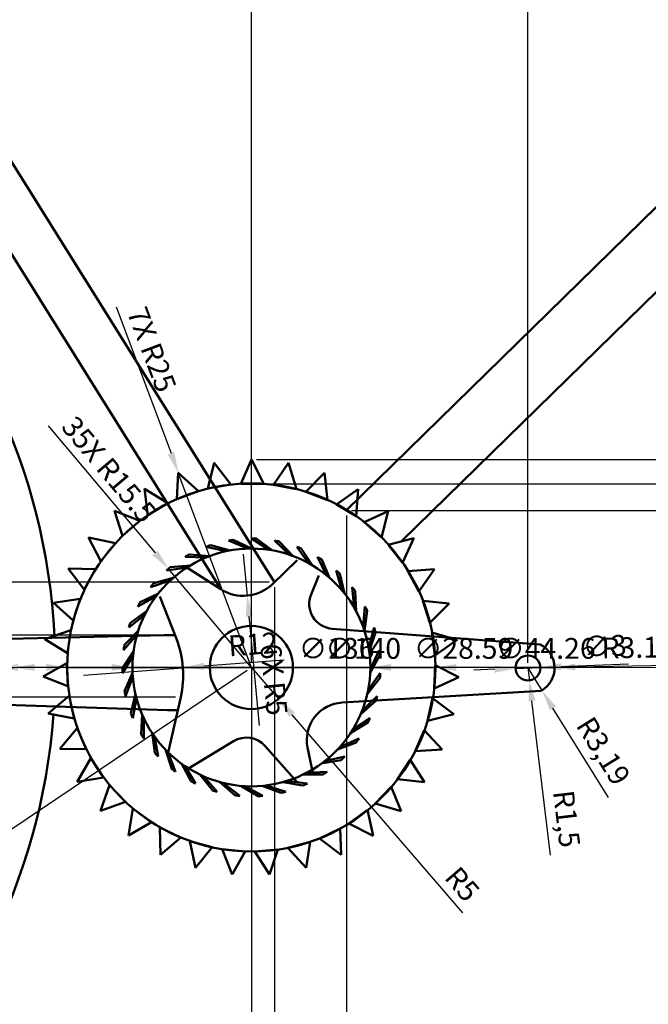
# Model space of a CAD drawing. Units: millimetres. Extents: x 1068 to 1546, y 1743 to 2032.
# Tile 4 of 9: x 1243 to 1318, y 1809 to 1928. Entities that reach past the tile are written whole.
import ezdxf

# ---------------------------------------------------------------- set-up
doc = ezdxf.new("R2010")
doc.units = ezdxf.units.MM
for name, color, linetype, lineweight in [('M-CONS', 8, 'Continuous', 18), ('M-DIMS', 2, 'Continuous', 25), ('M-OUTL', 7, 'Continuous', 50)]:
    doc.layers.add(name, color=color, linetype=linetype, lineweight=lineweight)
doc.styles.get("Standard").update_dxf_attribs({"font": 'arial.ttf'})
doc.dimstyles.new('ISO-25', dxfattribs={"dimtxt": 2.5, "dimasz": 2.5, "dimexe": 1.25, "dimexo": 0.625, "dimtad": 1, "dimtxsty": 'Standard', "dimcen": 2.5, "dimadec": 0, "dimazin": 0, "dimtfac": 1, "dimtmove": 0, "dimatfit": 3, "dimfxl": 1, "dimarcsym": 0})

# ---------------------------------------------------------------- blocks, each defined once
blk = doc.blocks.new('*U1')
for p, q in [((-1.39, -1.45), (-0.1, 1.46)), ((-0.1, 1.46), (1.39, -1.46)), ((1.39, -1.46), (-1.39, -1.45))]:
    blk.add_line(p, q)
blk = doc.blocks.new('*U2')
at = {"layer": 'M-OUTL', "color": 0, "linetype": 'ByBlock', "lineweight": -2, "transparency": 16777216}
for p, rotation in [((1266.68, 1872.95), 10.28571428571424), ((1275.09, 1872.9), 349.7142857142858), ((1262.61, 1871.85), 20.57142857142856), ((1279.15, 1871.75), 339.4285714285715), ((1258.79, 1870.04), 30.85714285714287), ((1282.94, 1869.9), 329.1428571428572), ((1255.37, 1867.58), 41.14285714285714), ((1286.34, 1867.4), 318.8571428571429), ((1252.43, 1864.54), 51.42857142857144), ((1289.24, 1864.33), 308.5714285714286), ((1250.09, 1861.04), 61.71428571428574), ((1291.54, 1860.8), 298.2857142857143), ((1248.41, 1857.16), 72.00000000000001), ((1293.18, 1856.91), 288), ((1247.44, 1853.06), 82.2857142857143), ((1294.1, 1852.79), 277.7142857142857), ((1247.23, 1848.84), 92.57142857142858), ((1294.26, 1848.57), 267.4285714285714), ((1247.77, 1844.66), 102.8571428571429), ((1293.67, 1844.39), 257.1428571428572), ((1249.05, 1840.63), 113.1428571428571), ((1292.34, 1840.39), 246.8571428571429), ((1251.03, 1836.91), 123.4285714285714), ((1290.32, 1836.68), 236.5714285714286), ((1253.64, 1833.59), 133.7142857142857), ((1287.67, 1833.4), 226.2857142857143), ((1256.81, 1830.8), 144), ((1284.48, 1830.64), 216), ((1260.42, 1828.61), 154.2857142857143), ((1280.84, 1828.5), 205.7142857142857), ((1264.36, 1827.11), 164.5714285714286), ((1268.51, 1826.33), 174.8571428571429), ((1276.88, 1827.04), 195.4285714285714), ((1272.73, 1826.31), 185.1428571428572)]:
    blk.add_blockref('*U1', p, dxfattribs=dict(at, rotation=rotation))
blk.add_blockref('*U1', (1270.89, 1873.3), dxfattribs=at)
blk = doc.blocks.new('*U3')
for p, q in [((0.05, -0.53), (-2.13, 0.52)), ((0.05, 0.68), (2.13, -0.68))]:
    blk.add_line(p, q)
blk = doc.blocks.new('*U4')
at = {"layer": 'M-OUTL', "color": 0, "linetype": 'ByBlock', "lineweight": -2, "transparency": 16777216}
for p, rotation in [((1265.53, 1863.62), 20.57142857142856), ((1268.09, 1864.34), 10.28571428571424), ((1273.38, 1864.36), 349.7142857142858), ((1275.95, 1863.66), 339.4285714285715), ((1263.14, 1862.46), 30.85714285714285), ((1278.34, 1862.51), 329.1428571428572), ((1261, 1860.89), 41.14285714285714), ((1280.5, 1860.96), 318.8571428571429), ((1259.17, 1858.96), 51.42857142857142), ((1282.34, 1859.04), 308.5714285714286), ((1257.71, 1856.74), 61.71428571428571), ((1283.81, 1856.83), 298.2857142857143), ((1256.67, 1854.29), 72), ((1284.87, 1854.39), 288), ((1285.47, 1851.8), 277.7142857142858), ((1256.09, 1851.7), 82.28571428571429), ((1255.98, 1849.05), 92.57142857142856), ((1285.6, 1849.15), 267.4285714285714), ((1256.35, 1846.41), 102.8571428571428), ((1285.25, 1846.51), 257.1428571428571), ((1257.18, 1843.89), 113.1428571428571), ((1284.44, 1843.98), 246.8571428571429), ((1258.45, 1841.55), 123.4285714285714), ((1283.19, 1841.64), 236.5714285714286), ((1260.11, 1839.48), 133.7142857142857), ((1281.54, 1839.56), 226.2857142857143), ((1262.12, 1837.74), 144), ((1279.54, 1837.8), 216), ((1264.4, 1836.39), 154.2857142857143), ((1277.26, 1836.43), 205.7142857142857), ((1266.89, 1835.46), 164.5714285714286), ((1274.78, 1835.49), 195.4285714285714), ((1269.51, 1835), 174.8571428571429), ((1272.17, 1835.01), 185.1428571428571)]:
    blk.add_blockref('*U3', p, dxfattribs=dict(at, rotation=rotation))
blk.add_blockref('*U3', (1270.74, 1864.58), dxfattribs=at)
blk = doc.blocks.new('*D5')
at = {"layer": 'Defpoints', "color": 0, "transparency": 16777216}
for p in [(1177.23, 1849.76), (1402.23, 1849.76), (1402.23, 1747.98)]:
    blk.add_point(p, dxfattribs=at)
at = {"layer": 'M-DIMS', "color": 0, "lineweight": -2, "transparency": 16777216}
for p, q in [((1177.23, 1849.14), (1177.23, 1746.73)), ((1402.23, 1849.14), (1402.23, 1746.73)), ((1179.73, 1747.98), (1399.73, 1747.98))]:
    blk.add_line(p, q, dxfattribs=at)
at = {"layer": 'M-DIMS', "color": 0, "transparency": 16777216}
for points in [[(1179.73, 1748.39), (1179.73, 1747.56), (1177.23, 1747.98)], [(1399.73, 1748.39), (1399.73, 1747.56), (1402.23, 1747.98)]]:
    blk.add_solid(points, dxfattribs=at)
at = {"layer": 'M-DIMS', "color": 0, "transparency": 16777216, "insert": (1289.73, 1749.88), "char_height": 2.5, "attachment_point": 5}
blk.add_mtext('225', dxfattribs=at)
blk = doc.blocks.new('*D6')
at = {"layer": 'Defpoints', "color": 0, "transparency": 16777216}
for p in [(1172.23, 1849.76), (1270.79, 1849.76), (1270.79, 1762.16)]:
    blk.add_point(p, dxfattribs=at)
at = {"layer": 'M-DIMS', "color": 0, "lineweight": -2, "transparency": 16777216}
for p, q in [((1172.23, 1849.14), (1172.23, 1760.91)), ((1270.79, 1849.14), (1270.79, 1760.91)), ((1174.73, 1762.16), (1268.29, 1762.16))]:
    blk.add_line(p, q, dxfattribs=at)
at = {"layer": 'M-DIMS', "color": 0, "transparency": 16777216}
for points in [[(1174.73, 1762.57), (1174.73, 1761.74), (1172.23, 1762.16)], [(1268.29, 1762.57), (1268.29, 1761.74), (1270.79, 1762.16)]]:
    blk.add_solid(points, dxfattribs=at)
at = {"layer": 'M-DIMS', "color": 0, "transparency": 16777216, "insert": (1221.51, 1764.28), "char_height": 2.5, "attachment_point": 5}
blk.add_mtext('98,56', dxfattribs=at)
blk = doc.blocks.new('*D18')
at = {"layer": 'Defpoints', "color": 0, "transparency": 16777216}
for p in [(1270.79, 1849.76), (1274.05, 1845.97)]:
    blk.add_point(p, dxfattribs=at)
at = {"layer": 'M-DIMS', "color": 0, "lineweight": -2, "transparency": 16777216}
for p, q in [((1270.79, 1849.76), (1274.05, 1845.97)), ((1296.19, 1820.25), (1275.68, 1844.08))]:
    blk.add_line(p, q, dxfattribs=at)
at = {"layer": 'M-DIMS', "color": 0, "transparency": 16777216}
blk.add_solid([(1276, 1844.35), (1275.36, 1843.81), (1274.05, 1845.97)], dxfattribs=at)
at = {"layer": 'M-DIMS', "color": 0, "transparency": 16777216, "insert": (1295.89, 1823.5), "char_height": 2.5, "attachment_point": 5, "rotation": 310.7194}
blk.add_mtext('R5', dxfattribs=at)
blk = doc.blocks.new('*D19')
at = {"layer": 'Defpoints', "color": 0, "transparency": 16777216}
for p in [(1304.02, 1849.7), (1304.2, 1848.21)]:
    blk.add_point(p, dxfattribs=at)
at = {"layer": 'M-DIMS', "color": 0, "lineweight": -2, "transparency": 16777216}
for p, q in [((1304.02, 1849.7), (1304.2, 1848.21)), ((1306.74, 1827.19), (1304.5, 1845.73))]:
    blk.add_line(p, q, dxfattribs=at)
at = {"layer": 'M-DIMS', "color": 0, "transparency": 16777216}
blk.add_solid([(1304.92, 1845.78), (1304.09, 1845.68), (1304.2, 1848.21)], dxfattribs=at)
at = {"layer": 'M-DIMS', "color": 0, "transparency": 16777216, "insert": (1308.36, 1831.52), "char_height": 2.5, "attachment_point": 5, "rotation": 276.8719}
blk.add_mtext('R1,5', dxfattribs=at)
blk = doc.blocks.new('*D20')
at = {"layer": 'Defpoints', "color": 0, "transparency": 16777216}
for p in [(1304.02, 1849.7), (1305.71, 1846.99)]:
    blk.add_point(p, dxfattribs=at)
at = {"layer": 'M-DIMS', "color": 0, "lineweight": -2, "transparency": 16777216}
for p, q in [((1304.02, 1849.7), (1305.71, 1846.99)), ((1313.69, 1834.12), (1307.02, 1844.86))]:
    blk.add_line(p, q, dxfattribs=at)
at = {"layer": 'M-DIMS', "color": 0, "transparency": 16777216}
blk.add_solid([(1307.38, 1845.08), (1306.67, 1844.64), (1305.71, 1846.99)], dxfattribs=at)
at = {"layer": 'M-DIMS', "color": 0, "transparency": 16777216, "insert": (1312.82, 1839.55), "char_height": 2.5, "attachment_point": 5, "rotation": 301.802}
blk.add_mtext('R3,19', dxfattribs=at)
blk = doc.blocks.new('*D23')
at = {"layer": 'Defpoints', "color": 0, "transparency": 16777216}
for p in [(1170.51, 1998.5), (1125.92, 1968.44), (1270.79, 1849.76)]:
    blk.add_point(p, dxfattribs=at)
at = {"layer": 'M-DIMS', "color": 0, "lineweight": -2, "transparency": 16777216}
for p, q in [((1169.99, 1998.15), (1124.89, 1967.74)), ((1224.8, 1821.77), (1127.32, 1966.36)), ((1270.27, 1849.41), (1225.16, 1819))]:
    blk.add_line(p, q, dxfattribs=at)
at = {"layer": 'M-DIMS', "color": 0, "transparency": 16777216}
for points in [[(1127.67, 1966.6), (1126.98, 1966.13), (1125.92, 1968.44)], [(1225.15, 1822.01), (1224.45, 1821.54), (1226.2, 1819.7)]]:
    blk.add_solid(points, dxfattribs=at)
at = {"layer": 'M-DIMS', "color": 0, "transparency": 16777216, "insert": (1177.82, 1895.26), "char_height": 2.5, "attachment_point": 5, "rotation": 303.9872}
blk.add_mtext('179,38', dxfattribs=at)
blk = doc.blocks.new('*D24')
at = {"layer": 'Defpoints', "color": 0, "transparency": 16777216}
for p in [(1270.79, 1850.31), (1402.23, 1850.31), (1402.23, 1761.81)]:
    blk.add_point(p, dxfattribs=at)
at = {"layer": 'M-DIMS', "color": 0, "lineweight": -2, "transparency": 16777216}
for p, q in [((1270.79, 1849.68), (1270.79, 1760.56)), ((1402.23, 1849.68), (1402.23, 1760.56)), ((1273.29, 1761.81), (1399.73, 1761.81))]:
    blk.add_line(p, q, dxfattribs=at)
at = {"layer": 'M-DIMS', "color": 0, "transparency": 16777216}
for points in [[(1273.29, 1762.23), (1273.29, 1761.4), (1270.79, 1761.81)], [(1399.73, 1762.23), (1399.73, 1761.4), (1402.23, 1761.81)]]:
    blk.add_solid(points, dxfattribs=at)
at = {"layer": 'M-DIMS', "color": 0, "transparency": 16777216, "insert": (1336.51, 1763.94), "char_height": 2.5, "attachment_point": 5}
blk.add_mtext('131,44', dxfattribs=at)
blk = doc.blocks.new('*D26')
at = {"layer": 'Defpoints', "color": 0, "transparency": 16777216}
for p in [(1304.02, 2028.2), (1270.79, 1849.76), (1304.02, 1849.7)]:
    blk.add_point(p, dxfattribs=at)
at = {"layer": 'M-DIMS', "color": 0, "lineweight": -2, "transparency": 16777216}
for p, q in [((1270.79, 1850.39), (1270.79, 2029.45)), ((1304.02, 1850.33), (1304.02, 2029.45)), ((1273.29, 2028.2), (1301.52, 2028.2))]:
    blk.add_line(p, q, dxfattribs=at)
at = {"layer": 'M-DIMS', "color": 0, "transparency": 16777216}
for points in [[(1273.29, 2028.61), (1273.29, 2027.78), (1270.79, 2028.2)], [(1301.52, 2028.61), (1301.52, 2027.78), (1304.02, 2028.2)]]:
    blk.add_solid(points, dxfattribs=at)
at = {"layer": 'M-DIMS', "color": 0, "transparency": 16777216, "insert": (1287.41, 2030.1), "char_height": 2.5, "attachment_point": 5}
blk.add_mtext('33.24', dxfattribs=at)
blk = doc.blocks.new('*D27')
at = {"layer": 'Defpoints', "color": 0, "transparency": 16777216}
for p in [(1270.79, 1874.76), (1507.48, 1874.76), (1272.28, 1871.84)]:
    blk.add_point(p, dxfattribs=at)
at = {"layer": 'M-DIMS', "color": 0, "lineweight": -2, "transparency": 16777216}
for p, q in [((1507.48, 1877.26), (1507.48, 1887.52)), ((1271.41, 1874.76), (1508.73, 1874.76)), ((1507.48, 1871.84), (1507.48, 1874.76)), ((1272.9, 1871.84), (1508.73, 1871.84)), ((1507.48, 1869.34), (1507.48, 1866.84))]:
    blk.add_line(p, q, dxfattribs=at)
at = {"layer": 'M-DIMS', "color": 0, "transparency": 16777216}
for points in [[(1507.06, 1877.26), (1507.89, 1877.26), (1507.48, 1874.76)], [(1507.06, 1869.34), (1507.89, 1869.34), (1507.48, 1871.84)]]:
    blk.add_solid(points, dxfattribs=at)
at = {"layer": 'M-DIMS', "color": 0, "transparency": 16777216, "insert": (1505.58, 1883.64), "char_height": 2.5, "attachment_point": 5, "rotation": 90}
blk.add_mtext('2.92', dxfattribs=at)
blk = doc.blocks.new('*D45')
at = {"layer": 'Defpoints', "color": 0, "transparency": 16777216}
for p in [(1212.56, 1957.56), (1273.55, 1860.03), (1273.55, 1744.51)]:
    blk.add_point(p, dxfattribs=at)
at = {"layer": 'M-DIMS', "color": 0, "lineweight": -2, "transparency": 16777216}
for p, q in [((1212.56, 1956.94), (1212.56, 1743.26)), ((1273.55, 1859.4), (1273.55, 1743.26)), ((1215.06, 1744.51), (1271.05, 1744.51))]:
    blk.add_line(p, q, dxfattribs=at)
at = {"layer": 'M-DIMS', "color": 0, "transparency": 16777216}
for points in [[(1215.06, 1744.93), (1215.06, 1744.1), (1212.56, 1744.51)], [(1271.05, 1744.93), (1271.05, 1744.1), (1273.55, 1744.51)]]:
    blk.add_solid(points, dxfattribs=at)
at = {"layer": 'M-DIMS', "color": 0, "transparency": 16777216, "insert": (1243.05, 1746.41), "char_height": 2.5, "attachment_point": 5}
blk.add_mtext('60.99', dxfattribs=at)
blk = doc.blocks.new('*D46')
at = {"layer": 'Defpoints', "color": 0, "transparency": 16777216}
for p in [(1212.56, 1957.56), (1071.98, 1860.03), (1273.55, 1860.03)]:
    blk.add_point(p, dxfattribs=at)
at = {"layer": 'M-DIMS', "color": 0, "lineweight": -2, "transparency": 16777216}
for p, q in [((1211.93, 1957.56), (1070.73, 1957.56)), ((1071.98, 1955.06), (1071.98, 1862.53)), ((1272.92, 1860.03), (1070.73, 1860.03))]:
    blk.add_line(p, q, dxfattribs=at)
at = {"layer": 'M-DIMS', "color": 0, "transparency": 16777216}
for points in [[(1071.57, 1955.06), (1072.4, 1955.06), (1071.98, 1957.56)], [(1071.57, 1862.53), (1072.4, 1862.53), (1071.98, 1860.03)]]:
    blk.add_solid(points, dxfattribs=at)
at = {"layer": 'M-DIMS', "color": 0, "transparency": 16777216, "insert": (1070.08, 1908.79), "char_height": 2.5, "attachment_point": 5, "rotation": 90}
blk.add_mtext('97.53', dxfattribs=at)
blk = doc.blocks.new('*D47')
at = {"layer": 'Defpoints', "color": 0, "transparency": 16777216}
for p in [(1361.34, 1946.14), (1282.2, 1868.65), (1361.34, 1744.51)]:
    blk.add_point(p, dxfattribs=at)
at = {"layer": 'M-DIMS', "color": 0, "lineweight": -2, "transparency": 16777216}
for p, q in [((1361.34, 1945.51), (1361.34, 1743.26)), ((1282.2, 1868.03), (1282.2, 1743.26)), ((1284.7, 1744.51), (1358.84, 1744.51))]:
    blk.add_line(p, q, dxfattribs=at)
at = {"layer": 'M-DIMS', "color": 0, "transparency": 16777216}
for points in [[(1284.7, 1744.93), (1284.7, 1744.1), (1282.2, 1744.51)], [(1358.84, 1744.93), (1358.84, 1744.1), (1361.34, 1744.51)]]:
    blk.add_solid(points, dxfattribs=at)
at = {"layer": 'M-DIMS', "color": 0, "transparency": 16777216, "insert": (1321.77, 1746.41), "char_height": 2.5, "attachment_point": 5}
blk.add_mtext('79.14', dxfattribs=at)
blk = doc.blocks.new('*D48')
at = {"layer": 'Defpoints', "color": 0, "transparency": 16777216}
for p in [(1361.34, 1946.14), (1507.48, 1946.14), (1282.2, 1868.65)]:
    blk.add_point(p, dxfattribs=at)
at = {"layer": 'M-DIMS', "color": 0, "lineweight": -2, "transparency": 16777216}
for p, q in [((1361.96, 1946.14), (1508.73, 1946.14)), ((1507.48, 1871.15), (1507.48, 1943.64)), ((1282.82, 1868.65), (1508.73, 1868.65))]:
    blk.add_line(p, q, dxfattribs=at)
at = {"layer": 'M-DIMS', "color": 0, "transparency": 16777216}
for points in [[(1507.06, 1943.64), (1507.89, 1943.64), (1507.48, 1946.14)], [(1507.06, 1871.15), (1507.89, 1871.15), (1507.48, 1868.65)]]:
    blk.add_solid(points, dxfattribs=at)
at = {"layer": 'M-DIMS', "color": 0, "transparency": 16777216, "insert": (1505.58, 1907.39), "char_height": 2.5, "attachment_point": 5, "rotation": 90}
blk.add_mtext('77.49', dxfattribs=at)
blk = doc.blocks.new('*D50')
at = {"layer": 'Defpoints', "color": 0, "transparency": 16777216}
for p in [(1261.6, 1853.65), (1071.98, 1846.18), (1262.3, 1846.18)]:
    blk.add_point(p, dxfattribs=at)
at = {"layer": 'M-DIMS', "color": 0, "lineweight": -2, "transparency": 16777216}
for p, q in [((1260.97, 1853.65), (1070.73, 1853.65)), ((1071.98, 1851.15), (1071.98, 1848.68)), ((1261.67, 1846.18), (1070.73, 1846.18)), ((1071.98, 1846.18), (1071.98, 1834.5))]:
    blk.add_line(p, q, dxfattribs=at)
at = {"layer": 'M-DIMS', "color": 0, "transparency": 16777216}
for points in [[(1071.57, 1851.15), (1072.4, 1851.15), (1071.98, 1853.65)], [(1071.57, 1848.68), (1072.4, 1848.68), (1071.98, 1846.18)]]:
    blk.add_solid(points, dxfattribs=at)
at = {"layer": 'M-DIMS', "color": 0, "transparency": 16777216, "insert": (1070.1, 1839.09), "char_height": 2.5, "attachment_point": 5, "rotation": 90}
blk.add_mtext('7.471', dxfattribs=at)
blk = doc.blocks.new('*D58')
at = {"layer": 'Defpoints', "color": 0, "transparency": 16777216}
for p in [(1102.23, 1849.76), (1242.23, 1849.76)]:
    blk.add_point(p, dxfattribs=at)
at = {"layer": 'M-DIMS', "color": 0, "lineweight": -2, "transparency": 16777216}
for p, q in [((1099.73, 1849.76), (1097.23, 1849.76)), ((1102.23, 1849.76), (1242.23, 1849.76)), ((1288.97, 1849.76), (1244.73, 1849.76))]:
    blk.add_line(p, q, dxfattribs=at)
at = {"layer": 'M-DIMS', "color": 0, "transparency": 16777216}
for points in [[(1099.73, 1850.18), (1099.73, 1849.35), (1102.23, 1849.76)], [(1244.73, 1850.18), (1244.73, 1849.35), (1242.23, 1849.76)]]:
    blk.add_solid(points, dxfattribs=at)
at = {"layer": 'M-DIMS', "color": 0, "transparency": 16777216, "insert": (1284.23, 1851.73), "char_height": 2.5, "attachment_point": 5, "rotation": 359.9997}
blk.add_mtext('∅140', dxfattribs=at)
blk = doc.blocks.new('*D59')
at = {"layer": 'Defpoints', "color": 0, "transparency": 16777216}
for p in [(1104.23, 1849.76), (1240.23, 1849.76)]:
    blk.add_point(p, dxfattribs=at)
at = {"layer": 'M-DIMS', "color": 0, "lineweight": -2, "transparency": 16777216}
for p, q in [((1101.73, 1849.76), (1099.23, 1849.76)), ((1104.23, 1849.76), (1240.23, 1849.76)), ((1285.77, 1849.76), (1242.73, 1849.76))]:
    blk.add_line(p, q, dxfattribs=at)
at = {"layer": 'M-DIMS', "color": 0, "transparency": 16777216}
for points in [[(1101.73, 1850.18), (1101.73, 1849.35), (1104.23, 1849.76)], [(1242.73, 1850.18), (1242.73, 1849.35), (1240.23, 1849.76)]]:
    blk.add_solid(points, dxfattribs=at)
at = {"layer": 'M-DIMS', "color": 0, "transparency": 16777216, "insert": (1281.03, 1851.73), "char_height": 2.5, "attachment_point": 5, "rotation": 359.9997}
blk.add_mtext('∅136', dxfattribs=at)
blk = doc.blocks.new('*D62')
at = {"layer": 'Defpoints', "color": 0, "transparency": 16777216}
for p in [(1248.66, 1849.76), (1292.92, 1849.76)]:
    blk.add_point(p, dxfattribs=at)
at = {"layer": 'M-DIMS', "color": 0, "lineweight": -2, "transparency": 16777216}
for p, q in [((1246.16, 1849.76), (1243.66, 1849.76)), ((1248.66, 1849.76), (1292.92, 1849.76)), ((1312.4, 1849.76), (1295.42, 1849.76))]:
    blk.add_line(p, q, dxfattribs=at)
at = {"layer": 'M-DIMS', "color": 0, "transparency": 16777216}
for points in [[(1246.16, 1850.18), (1246.16, 1849.35), (1248.66, 1849.76)], [(1295.42, 1850.18), (1295.42, 1849.35), (1292.92, 1849.76)]]:
    blk.add_solid(points, dxfattribs=at)
at = {"layer": 'M-DIMS', "color": 0, "transparency": 16777216, "insert": (1306.19, 1851.73), "char_height": 2.5, "attachment_point": 5, "rotation": 359.9992}
blk.add_mtext('∅44.26', dxfattribs=at)
blk = doc.blocks.new('*D63')
at = {"layer": 'Defpoints', "color": 0, "transparency": 16777216}
for p in [(1256.49, 1849.76), (1285.08, 1849.76)]:
    blk.add_point(p, dxfattribs=at)
at = {"layer": 'M-DIMS', "color": 0, "lineweight": -2, "transparency": 16777216}
for p, q in [((1253.99, 1849.76), (1251.49, 1849.76)), ((1256.49, 1849.76), (1285.08, 1849.76)), ((1302.49, 1849.76), (1287.58, 1849.76))]:
    blk.add_line(p, q, dxfattribs=at)
at = {"layer": 'M-DIMS', "color": 0, "transparency": 16777216}
for points in [[(1253.99, 1850.18), (1253.99, 1849.35), (1256.49, 1849.76)], [(1287.58, 1850.18), (1287.58, 1849.35), (1285.08, 1849.76)]]:
    blk.add_solid(points, dxfattribs=at)
at = {"layer": 'M-DIMS', "color": 0, "transparency": 16777216, "insert": (1296.29, 1851.73), "char_height": 2.5, "attachment_point": 5, "rotation": 359.9987}
blk.add_mtext('∅28.59', dxfattribs=at)
blk = doc.blocks.new('*D64')
at = {"layer": 'Defpoints', "color": 0, "transparency": 16777216}
for p in [(1262, 1873.17), (1270.79, 1849.76)]:
    blk.add_point(p, dxfattribs=at)
at = {"layer": 'M-DIMS', "color": 0, "lineweight": -2, "transparency": 16777216}
for p, q in [((1254.52, 1893.11), (1261.13, 1875.51)), ((1270.79, 1849.76), (1262, 1873.17))]:
    blk.add_line(p, q, dxfattribs=at)
at = {"layer": 'M-DIMS', "color": 0, "transparency": 16777216}
blk.add_solid([(1261.52, 1875.66), (1260.74, 1875.36), (1262, 1873.17)], dxfattribs=at)
at = {"layer": 'M-DIMS', "color": 0, "transparency": 16777216, "insert": (1258.52, 1887.88), "char_height": 2.5, "attachment_point": 5, "rotation": 290.5657}
blk.add_mtext('7X R25', dxfattribs=at)
blk = doc.blocks.new('*D67')
at = {"layer": 'Defpoints', "color": 0, "transparency": 16777216}
for p in [(1260.82, 1861.63), (1270.79, 1849.76)]:
    blk.add_point(p, dxfattribs=at)
at = {"layer": 'M-DIMS', "color": 0, "lineweight": -2, "transparency": 16777216}
for p, q in [((1246.36, 1878.83), (1259.21, 1863.54)), ((1270.79, 1849.76), (1260.82, 1861.63))]:
    blk.add_line(p, q, dxfattribs=at)
at = {"layer": 'M-DIMS', "color": 0, "transparency": 16777216}
blk.add_solid([(1259.53, 1863.81), (1258.89, 1863.27), (1260.82, 1861.63)], dxfattribs=at)
at = {"layer": 'M-DIMS', "color": 0, "transparency": 16777216, "insert": (1253.44, 1873.37), "char_height": 2.5, "attachment_point": 5, "rotation": 310.0415}
blk.add_mtext('35X R15.5', dxfattribs=at)
blk = doc.blocks.new('*D71')
at = {"layer": 'Defpoints', "color": 0, "transparency": 16777216}
for p in [(1262.56, 1849.72), (1250.6, 1848.84)]:
    blk.add_point(p, dxfattribs=at)
at = {"layer": 'M-DIMS', "color": 0, "lineweight": -2, "transparency": 16777216}
for p, q in [((1274.73, 1850.62), (1265.06, 1849.91)), ((1250.6, 1848.84), (1262.56, 1849.72))]:
    blk.add_line(p, q, dxfattribs=at)
at = {"layer": 'M-DIMS', "color": 0, "transparency": 16777216}
blk.add_solid([(1265.03, 1850.32), (1265.09, 1849.49), (1262.56, 1849.72)], dxfattribs=at)
at = {"layer": 'M-DIMS', "color": 0, "transparency": 16777216, "insert": (1271, 1852.23), "char_height": 2.5, "attachment_point": 5, "rotation": 4.2369}
blk.add_mtext('R12', dxfattribs=at)
blk = doc.blocks.new('*D77')
at = {"layer": 'Defpoints', "color": 0, "transparency": 16777216}
for p in [(1269.81, 1863.37), (1270.29, 1858.39)]:
    blk.add_point(p, dxfattribs=at)
at = {"layer": 'M-DIMS', "color": 0, "lineweight": -2, "transparency": 16777216}
for p, q in [((1269.81, 1863.37), (1270.29, 1858.39)), ((1271.78, 1842.78), (1270.53, 1855.91))]:
    blk.add_line(p, q, dxfattribs=at)
at = {"layer": 'M-DIMS', "color": 0, "transparency": 16777216}
blk.add_solid([(1270.94, 1855.95), (1270.11, 1855.87), (1270.29, 1858.39)], dxfattribs=at)
at = {"layer": 'M-DIMS', "color": 0, "transparency": 16777216, "insert": (1273.17, 1848.28), "char_height": 2.5, "attachment_point": 5, "rotation": 275.4682}
blk.add_mtext('6X R5', dxfattribs=at)
blk = doc.blocks.new('*D84')
at = {"layer": 'Defpoints', "color": 0, "transparency": 16777216}
for p in [(1302.52, 1849.64), (1305.52, 1849.76)]:
    blk.add_point(p, dxfattribs=at)
at = {"layer": 'M-DIMS', "color": 0, "lineweight": -2, "transparency": 16777216}
for p, q in [((1300.03, 1849.55), (1297.53, 1849.45)), ((1302.52, 1849.64), (1305.52, 1849.76)), ((1316.12, 1850.16), (1308.02, 1849.85))]:
    blk.add_line(p, q, dxfattribs=at)
at = {"layer": 'M-DIMS', "color": 0, "transparency": 16777216}
for points in [[(1300.01, 1849.97), (1300.04, 1849.13), (1302.52, 1849.64)], [(1308.01, 1850.27), (1308.04, 1849.44), (1305.52, 1849.76)]]:
    blk.add_solid(points, dxfattribs=at)
at = {"layer": 'M-DIMS', "color": 0, "transparency": 16777216, "insert": (1313.25, 1852.03), "char_height": 2.5, "attachment_point": 5, "rotation": 2.1836}
blk.add_mtext('∅3', dxfattribs=at)
blk = doc.blocks.new('*D85')
at = {"layer": 'Defpoints', "color": 0, "transparency": 16777216}
for p in [(1304.02, 1849.7), (1307.22, 1849.76)]:
    blk.add_point(p, dxfattribs=at)
at = {"layer": 'M-DIMS', "color": 0, "lineweight": -2, "transparency": 16777216}
for p, q in [((1304.02, 1849.7), (1307.22, 1849.76)), ((1324.27, 1850.07), (1309.71, 1849.81))]:
    blk.add_line(p, q, dxfattribs=at)
at = {"layer": 'M-DIMS', "color": 0, "transparency": 16777216}
blk.add_solid([(1309.71, 1850.22), (1309.72, 1849.39), (1307.22, 1849.76)], dxfattribs=at)
at = {"layer": 'M-DIMS', "color": 0, "transparency": 16777216, "insert": (1318.21, 1851.86), "char_height": 2.5, "attachment_point": 5, "rotation": 1.0509}
blk.add_mtext('R3.192', dxfattribs=at)

msp = doc.modelspace()

# ---------------------------------------------------------------- linework, layer by layer
at = {"layer": 'M-CONS'}
for q in [(1402.2281, 1849.7623), (1270.787, 1849.7623)]:
    msp.add_line((1172.2281, 1849.7623), q, dxfattribs=at)
at = {"layer": 'M-OUTL'}
for p, q in [((1272.1243, 1862.3034), (1199.166, 1978.9798)), ((1282.1954, 1868.6519), (1361.339, 1946.1377)), ((1267.1078, 1859.1666), (1215.8973, 1941.0634)), ((1288.8124, 1864.9272), (1365.2237, 1939.738)), ((1287.7439, 1863.8811), (1287.7894, 1863.9256)), ((1272.1243, 1862.3034), (1273.5484, 1860.0259)), ((1273.2665, 1859.7565), (1276.289, 1862.6441)), ((1263.0454, 1861.7795), (1267.1078, 1859.1666)), ((1278.9071, 1860.8385), (1277.9635, 1858.5488)), ((1261.7811, 1853.1844), (1259.7946, 1858.293)), ((1280.512, 1854.4141), (1305.4963, 1852.5341)), ((1176.8658, 1851.631), (1260.3118, 1853.653)), ((1260.3118, 1853.653), (1261.5989, 1853.653)), ((1176.626, 1847.3836), (1260.7126, 1844.644)), ((1281.6856, 1845.5358), (1305.6181, 1846.9364)), ((1260.7938, 1839.5408), (1262.2997, 1846.1816)), ((1260.7126, 1844.644), (1261.951, 1844.644)), ((1268.6426, 1840.8957), (1263.0298, 1837.5062)), ((1276.2824, 1835.958), (1272.4437, 1840.3117)), ((1278.1995, 1836.8826), (1277.538, 1840.1506))]:
    msp.add_line(p, q, dxfattribs=at)
for centre, radius in [((1270.787, 1849.7623), 22.1287), ((1270.787, 1849.7623), 22.1287), ((1270.787, 1849.7623), 14.2949), ((1270.787, 1849.7623), 5), ((1304.0238, 1849.7019), 1.5)]:
    msp.add_circle(centre, radius, dxfattribs=at)
for centre, radius, start, end in [((1172.2281, 1849.7623), 75, 2.898254, 355.67622), ((1270.787, 1849.7623), 25, 100.277187, 100.290732), ((1270.787, 1849.7623), 25, 110.552087, 110.578742), ((1270.787, 1849.7623), 25, 120.825046, 120.863956), ((1270.787, 1849.7623), 25, 131.096473, 131.14639), ((1270.787, 1849.7623), 25, 141.366828, 141.42615), ((1270.787, 1849.7623), 15.5, 98.086319, 100.285714), ((1270.787, 1849.7623), 15.5, 87.800605, 90), ((1270.787, 1849.7623), 15.5, 77.514891, 79.714286), ((1270.787, 1849.7623), 15.5, 108.372033, 110.571429), ((1270.787, 1849.7623), 15.5, 67.229176, 69.428571), ((1270.787, 1849.7623), 15.5, 118.657748, 120.857143), ((1270.787, 1849.7623), 15.5, 56.943462, 59.142857), ((1270.787, 1849.7623), 25, 151.636603, 151.703427), ((1270.787, 1849.7623), 15.5, 128.943462, 131.142857), ((1270.787, 1849.7623), 15.5, 46.657748, 48.857143), ((1270.787, 1849.7623), 15.5, 139.229176, 141.428571), ((1269.8126, 1863.3718), 5, 237.251, 313.691982), ((1270.787, 1849.7623), 15.5, 36.372033, 38.571429), ((1270.787, 1849.7623), 15.5, 149.514891, 151.714286), ((1280.7371, 1857.4057), 3, 157.601851, 265.696722), ((1270.787, 1849.7623), 15.5, 26.086319, 28.285714), ((1270.787, 1849.7623), 15.5, 159.800605, 162), ((1270.787, 1849.7623), 15.5, 15.800605, 18), ((1270.787, 1849.7623), 25, 172.176467, 172.251692), ((1250.5968, 1848.8354), 12, 347.223179, 21.248332), ((1270.787, 1849.7623), 15.5, 170.086319, 172.285714), ((1270.787, 1849.7623), 15.5, 5.514891, 7.714286), ((1304.0238, 1849.7019), 3.1921, 299.963596, 62.529386), ((1270.787, 1849.7623), 15.5, 180.372033, 182.571429), ((1270.787, 1849.7623), 15.5, 355.229176, 357.428571), ((1270.787, 1849.7623), 15.5, 190.657748, 192.857143), ((1270.787, 1849.7623), 15.5, 344.943462, 347.142857), ((1281.9485, 1841.0434), 4.5, 93.349473, 191.443943), ((1270.787, 1849.7623), 15.5, 200.943462, 203.142857), ((1270.787, 1849.7623), 15.5, 334.657748, 336.857143), ((1270.787, 1849.7623), 15.5, 211.229176, 213.428571), ((1270.1934, 1838.3276), 3, 41.403198, 121.126698), ((1270.787, 1849.7623), 15.5, 324.372033, 326.571429), ((1270.787, 1849.7623), 15.5, 221.514891, 223.714286), ((1270.787, 1849.7623), 15.5, 314.086319, 316.285714), ((1270.787, 1849.7623), 15.5, 231.800605, 234), ((1270.787, 1849.7623), 15.5, 303.800605, 306), ((1270.787, 1849.7623), 15.5, 242.086319, 244.285714), ((1270.787, 1849.7623), 15.5, 293.514891, 295.714286), ((1270.787, 1849.7623), 15.5, 252.372033, 254.571429), ((1270.787, 1849.7623), 15.5, 262.657748, 264.857143), ((1270.787, 1849.7623), 15.5, 272.943462, 275.142857), ((1270.787, 1849.7623), 15.5, 283.229176, 285.428571)]:
    msp.add_arc(centre, radius, start, end, dxfattribs=at)

# ---------------------------------------------------------------- block references
for name in ['*U2', '*U4']:
    msp.add_blockref(name, (0, 0), dxfattribs=at)

# ---------------------------------------------------------------- dimensions: what is measured, and where the dimension line sits
at = {"layer": 'M-DIMS'}
for base, p1, p2, override, picture, middle in [((1304.0238, 2028.1976), (1270.787, 1849.7623), (1304.0238, 1849.7019), {"dimdec": 2, "dimlfac": 1, "dimrnd": 0, "dimzin": 0, "dimdsep": 46, "dimlunit": 2}, '*D26', (1287.4054, 2030.0999)), ((1273.5484, 1744.5123), (1212.5594, 1957.5607), (1273.5484, 1860.0259), {"dimdec": 2, "dimlfac": 1, "dimrnd": 0, "dimzin": 0, "dimdsep": 46, "dimlunit": 2}, '*D45', (1243.0539, 1746.4138)), ((1361.339, 1744.5123), (1282.1954, 1868.6519), (1361.339, 1946.1377), {"dimdec": 2, "dimlfac": 1, "dimrnd": 0, "dimzin": 0, "dimdsep": 46, "dimlunit": 2}, '*D47', (1321.7672, 1746.4138)), ((1270.787, 1762.1558), (1172.2281, 1849.7623), (1270.787, 1849.7623), {"dimclrd": 0, "dimclre": 0, "dimclrt": 0}, '*D6', (1221.5076, 1764.2832)), ((1402.2281, 1747.9766), (1177.2281, 1849.7623), (1402.2281, 1849.7623), {"dimclrd": 0, "dimclre": 0, "dimclrt": 0}, '*D5', (1289.7281, 1749.8781)), ((1402.2281, 1761.8125), (1270.787, 1850.3085), (1402.2281, 1850.3085), {"dimclrd": 0, "dimclre": 0, "dimclrt": 0}, '*D24', (1336.5076, 1763.9399))]:
    dim = msp.add_linear_dim(base=base, p1=p1, p2=p2, dimstyle='ISO-25', override=override, dxfattribs=at)
    dim.commit()
    dim.dimension.update_dxf_attribs({"geometry": picture, "text_midpoint": middle})
dim = msp.add_aligned_dim(p1=(1270.787, 1849.7623), p2=(1170.5128, 1998.4966), distance=53.7765, dimstyle='ISO-25', override={"dimclrd": 0, "dimclre": 0, "dimclrt": 0}, dxfattribs=at)
dim.commit()
dim.dimension.update_dxf_attribs({"geometry": '*D23', "text_midpoint": (1177.8244, 1895.2572)})
for base, p1, p2, override, picture, middle in [((1071.9839, 1860.0259), (1212.5594, 1957.5607), (1273.5484, 1860.0259), {"dimdec": 2, "dimlfac": 1, "dimrnd": 0, "dimzin": 0, "dimdsep": 46, "dimlunit": 2}, '*D46', (1070.0816, 1908.7933)), ((1507.4781, 1946.1377), (1282.1954, 1868.6519), (1361.339, 1946.1377), {"dimdec": 2, "dimlfac": 1, "dimrnd": 0, "dimzin": 0, "dimdsep": 46, "dimlunit": 2}, '*D48', (1505.5767, 1907.3948)), ((1507.4781, 1874.7623), (1272.2751, 1871.8409), (1270.787, 1874.7623), {"dimdec": 2, "dimlfac": 1, "dimrnd": 0, "dimzin": 0, "dimdsep": 46, "dimlunit": 2}, '*D27', (1505.5767, 1883.6428)), ((1071.9839, 1846.1816), (1261.5989, 1853.653), (1262.2997, 1846.1816), {"dimdec": 3, "dimlfac": 1, "dimrnd": 0, "dimzin": 0, "dimdsep": 46, "dimlunit": 2}, '*D50', (1070.1038, 1839.09))]:
    dim = msp.add_linear_dim(base=base, p1=p1, p2=p2, angle=90, dimstyle='ISO-25', override=override, dxfattribs=at)
    dim.commit()
    dim.dimension.update_dxf_attribs({"geometry": picture, "text_midpoint": middle})
dim = msp.add_radius_dim(center=(1270.787, 1849.7623), mpoint=(1262.005, 1873.1691), text='7X <>', dimstyle='ISO-25', override={"dimdec": 0, "dimlfac": 1, "dimrnd": 0, "dimzin": 0, "dimdsep": 46, "dimlunit": 2}, dxfattribs=at)
dim.commit()
dim.dimension.update_dxf_attribs({"geometry": '*D64', "text_midpoint": (1256.7358, 1887.2131), "dimtype": 164})
for center, mpoint, text, override, picture, middle in [((1270.787, 1849.7623), (1260.8152, 1861.6288), '35X <>', {"dimdec": 1, "dimlfac": 1, "dimrnd": 0, "dimzin": 0, "dimdsep": 46, "dimlunit": 2}, '*D67', (1253.436, 1873.3669)), ((1269.8126, 1863.3718), (1270.289, 1858.3946), '6X <>', {"dimdec": 0, "dimlfac": 1, "dimrnd": 0, "dimzin": 0, "dimdsep": 46, "dimlunit": 2}, '*D77', (1273.1674, 1848.2801))]:
    dim = msp.add_radius_dim(center=center, mpoint=mpoint, text=text, dimstyle='ISO-25', override=override, dxfattribs=at)
    dim.commit()
    dim.dimension.update_dxf_attribs({"geometry": picture, "text_midpoint": middle})
for center, mpoint, override, picture, middle in [((1250.5968, 1848.8354), (1262.5641, 1849.722), {"dimdec": 0, "dimlfac": 1, "dimrnd": 0, "dimzin": 0, "dimdsep": 46, "dimlunit": 2}, '*D71', (1271.0007, 1852.2323)), ((1304.0238, 1849.7019), (1307.2154, 1849.7604), {"dimdec": 3, "dimlfac": 1, "dimrnd": 0, "dimzin": 0, "dimdsep": 46, "dimlunit": 2}, '*D85', (1318.2052, 1851.8647)), ((1304.0238, 1849.7019), (1305.706, 1846.989), {"dimclrd": 0, "dimclre": 0, "dimclrt": 0}, '*D20', (1312.8212, 1839.5512))]:
    dim = msp.add_radius_dim(center=center, mpoint=mpoint, dimstyle='ISO-25', override=override, dxfattribs=at)
    dim.commit()
    dim.dimension.update_dxf_attribs({"geometry": picture, "text_midpoint": middle})
for p1, p2, override, picture, middle in [((1102.2281, 1849.7627), (1242.2281, 1849.762), {"dimdec": 0, "dimlfac": 1, "dimrnd": 0, "dimzin": 0, "dimdsep": 46, "dimlunit": 2}, '*D58', (1284.2281, 1849.7618)), ((1104.2281, 1849.7627), (1240.2281, 1849.762), {"dimdec": 0, "dimlfac": 1, "dimrnd": 0, "dimzin": 0, "dimdsep": 46, "dimlunit": 2}, '*D59', (1281.0281, 1849.7618)), ((1248.6583, 1849.7627), (1292.9157, 1849.762), {"dimdec": 2, "dimlfac": 1, "dimrnd": 0, "dimzin": 0, "dimdsep": 46, "dimlunit": 2}, '*D62', (1306.1929, 1849.7618)), ((1256.4921, 1849.7627), (1285.0818, 1849.762), {"dimdec": 2, "dimlfac": 1, "dimrnd": 0, "dimzin": 0, "dimdsep": 46, "dimlunit": 2}, '*D63', (1296.2875, 1849.7617))]:
    dim = msp.add_diameter_dim_2p(p1=p1, p2=p2, dimstyle='ISO-25', override=override, dxfattribs=at)
    dim.commit()
    dim.dimension.update_dxf_attribs({"geometry": picture, "text_midpoint": middle, "dimtype": 163})
dim = msp.add_diameter_dim_2p(p1=(1302.5249, 1849.6447), p2=(1305.5227, 1849.7591), dimstyle='ISO-25', override={"dimdec": 0, "dimlfac": 1, "dimrnd": 0, "dimzin": 0, "dimdsep": 46, "dimlunit": 2}, dxfattribs=at)
dim.commit()
dim.dimension.update_dxf_attribs({"geometry": '*D84', "text_midpoint": (1313.3215, 1850.0564)})
for center, mpoint, picture, middle in [((1270.787, 1849.7623), (1274.0488, 1845.9728), '*D18', (1294.4565, 1822.2629)), ((1304.0238, 1849.7019), (1304.2033, 1848.2127), '*D19', (1306.2458, 1831.2647))]:
    dim = msp.add_radius_dim(center=center, mpoint=mpoint, dimstyle='ISO-25', override={"dimclrd": 0, "dimclre": 0, "dimclrt": 0}, dxfattribs=at)
    dim.commit()
    dim.dimension.update_dxf_attribs({"geometry": picture, "text_midpoint": middle, "dimtype": 164})

doc.saveas('drawing.dxf')
